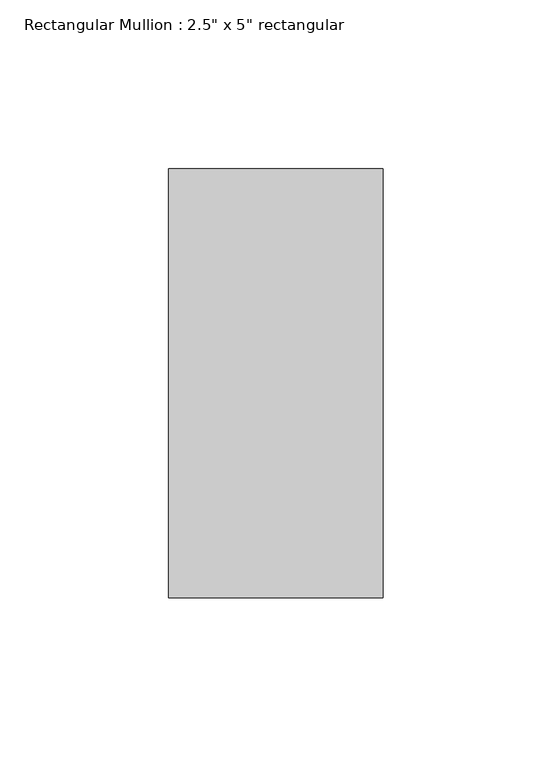
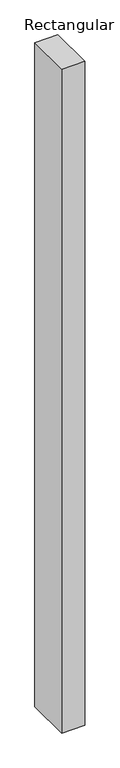
"""IFC4 building model written with IfcOpenShell, lengths in millimetres: member geometry."""

from ifc_helpers import new_model, si_unit, frame, origin, place, context, project, spatial, polyline, outline, extrude, source, transform, mapped, element, save


def member_9857a5fa(model_context):
    return source(origin(), model_context, "Body", "SweptSolid", [
        extrude(outline(polyline([(31.75, 63.5), (31.75, -63.5), (-31.75, -63.5), (-31.75, 63.5), (31.75, 63.5)])), frame((0.0, 0.0, -1931.193737), z_axis=(0.0, 0.0, 1.0), x_axis=(1.0, 0.0, 0.0)), (0.0, 0.0, 1.0), 1931.193737),
    ])


if __name__ == "__main__":
    model = new_model("IFC4")
    model_context = context("Model", 3, world=origin())
    ifc_project = project(units=[si_unit("LENGTHUNIT", "METRE", prefix="MILLI")], contexts=[model_context])
    site = spatial("IfcSite", under=ifc_project)
    building = spatial("IfcBuilding", under=site)
    placement = place(None, origin())
    member_shape = member_9857a5fa(model_context)
    element("IfcMember", 1, ObjectType="Rectangular Mullion : 2.5\" x 5\" rectangular", at=placement, inside=building, context=model_context, shape_type="MappedRepresentation", body=[
        mapped(member_shape, transform((0.0, 0.0, 0.0), x_axis=(1.0, 0.0, 0.0), y_axis=(0.0, 1.0, 0.0), z_axis=(0.0, 0.0, 1.0))),
    ])
    save(model, "model.ifc")

# Revit data of these elements
# Type "Rectangular Mullion : 2.5\" x 5\" rectangular"
#   built-in parameter 1007304 = 0.416667 (stored number, unit not read)
#   built-in parameter 1007301 = 0.104167 (stored number, unit not read)
#   built-in parameter 1007300 = 0.104167 (stored number, unit not read)
# Element 1 (IfcMember, "Rectangular Mullion : 2.5\" x 5\" rectangular")
#   Materials on its faces: "Aluminum"
# Materials
#   "Aluminum": class "Metal", colour RGB 247 247 247, transparency 0, Description = "Aluminum 6061", Cost = 0
